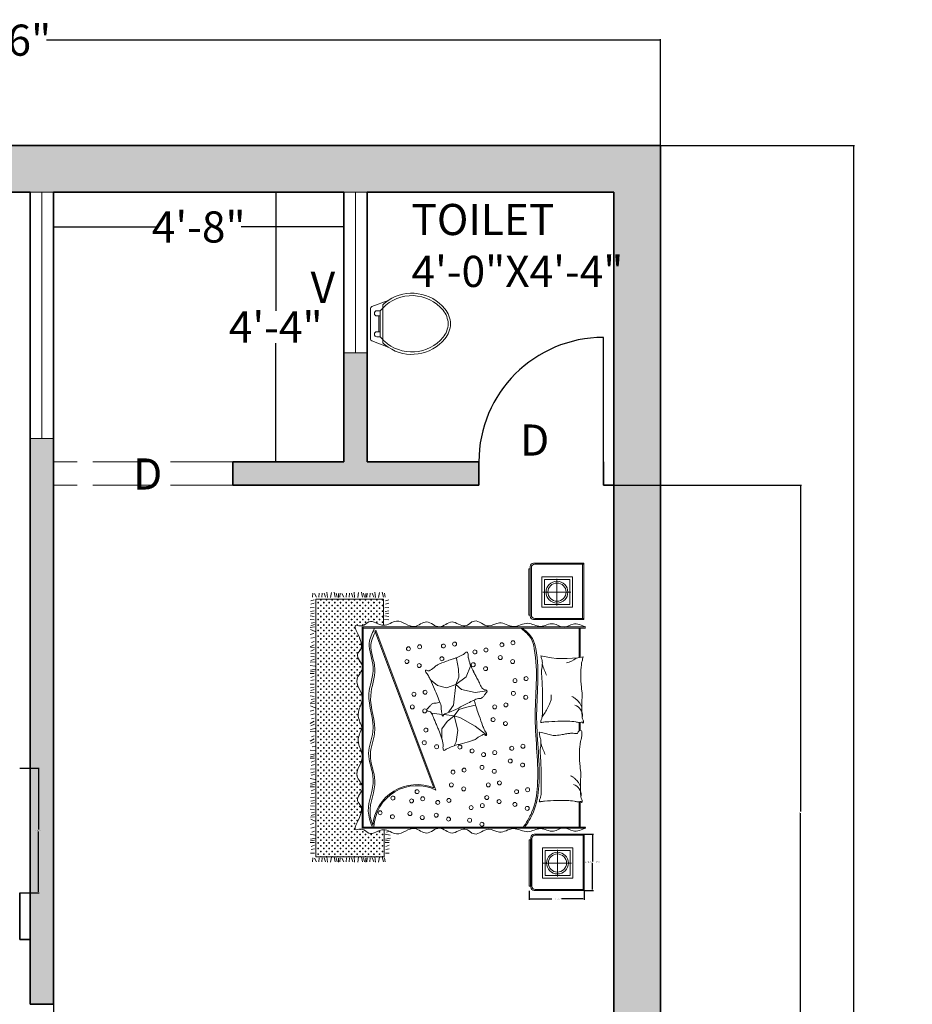
# Model space of a CAD drawing. Units: inches. Extents: x -5 to 330, y -522 to 40.
# Tile 23 of 23: x 158 to 330, y -153 to 37. Entities that reach past the tile are written whole.
import ezdxf

# ---------------------------------------------------------------- set-up
doc = ezdxf.new("R2010")
doc.units = ezdxf.units.IN
doc.header["$MEASUREMENT"] = 0
doc.linetypes.add('ACAD_ISO02W100', pattern=[15, 12, -3])
for name, color, linetype, lineweight in [('A-ANNO-DIMS', 2, 'Continuous', 18), ('A-ANNO-TEXT', 7, 'Continuous', 18), ('A-AREA-IDEN', 7, 'Continuous', 25), ('A-DOOR', 4, 'Continuous', 25), ('A-FURN', 8, 'Continuous', 18), ('A-FURN-PATT', 9, 'Continuous', 13), ('A-GLAZ', 4, 'Continuous', 18), ('A-WALL', 7, 'Continuous', 35), ('A-WALL-OVHD', 8, 'ACAD_ISO02W100', 18), ('WC-Detail_dwgmodels.com', 251, 'Continuous', 13), ('WC-Outline_dwgmodels.com', 250, 'Continuous', 18)]:
    doc.layers.add(name, color=color, linetype=linetype, lineweight=lineweight)
doc.layers.add('A-WALL-PATT', color=18, linetype='Continuous', lineweight=13, true_color=0x000000)
doc.styles.get("Standard").update_dxf_attribs({"font": 'arial.ttf'})
doc.dimstyles.get("Standard").update_dxf_attribs({"dimtxt": 0.18, "dimasz": 0.18, "dimexe": 0.18, "dimexo": 0.0625, "dimgap": 0.09, "dimtad": 0, "dimtih": 1, "dimtoh": 1, "dimdec": 0, "dimzin": 0, "dimdsep": 46, "dimlunit": 3, "dimtxsty": 'Standard', "dimcen": 0.09, "dimadec": 0, "dimazin": 0, "dimtfac": 1, "dimtdec": 0, "dimtofl": 0, "dimtmove": 0, "dimatfit": 3, "dimfxl": 1, "dimtolj": 1, "dimtzin": 0, "dimarcsym": 0})

# ---------------------------------------------------------------- blocks, each defined once
blk = doc.blocks.new('*D1')
at = {"layer": 'A-ANNO-DIMS', "color": 0, "lineweight": -2, "transparency": 16777216}
for p, q in [((23.51, 12.42), (23.51, 32.82)), ((23.69, 32.64), (141.81, 32.64)), ((280.83, 32.64), (162.71, 32.64)), ((281.01, 12.42), (281.01, 32.82))]:
    blk.add_line(p, q, dxfattribs=at)
at = {"layer": 'A-ANNO-DIMS', "color": 0, "transparency": 16777216}
for points in [[(23.69, 32.67), (23.69, 32.61), (23.51, 32.64)], [(280.83, 32.67), (280.83, 32.61), (281.01, 32.64)]]:
    blk.add_solid(points, dxfattribs=at)
at = {"layer": 'Defpoints', "color": 0, "transparency": 16777216}
for p in [(281.01, 32.64), (23.51, 12.36), (281.01, 12.36)]:
    blk.add_point(p, dxfattribs=at)
at = {"layer": 'A-ANNO-DIMS', "color": 0, "transparency": 16777216, "insert": (152.26, 32.64), "char_height": 6, "attachment_point": 5}
blk.add_mtext('\\A1;21\'-6"', dxfattribs=at)
blk = doc.blocks.new('*D6')
at = {"layer": 'A-ANNO-DIMS', "color": 0, "lineweight": -2, "transparency": 16777216}
for p, q in [((281.07, 12.36), (318.43, 12.36)), ((318.25, 12.18), (318.25, -238.29)), ((318.25, -494.96), (318.25, -244.5)), ((281.07, -495.14), (318.43, -495.14))]:
    blk.add_line(p, q, dxfattribs=at)
at = {"layer": 'A-ANNO-DIMS', "color": 0, "transparency": 16777216}
for points in [[(318.22, 12.18), (318.28, 12.18), (318.25, 12.36)], [(318.22, -494.96), (318.28, -494.96), (318.25, -495.14)]]:
    blk.add_solid(points, dxfattribs=at)
at = {"layer": 'Defpoints', "color": 0, "transparency": 16777216}
for p in [(281.01, 12.36), (281.01, -495.14), (318.25, -495.14)]:
    blk.add_point(p, dxfattribs=at)
at = {"layer": 'A-ANNO-DIMS', "color": 0, "transparency": 16777216, "insert": (318.25, -241.39), "char_height": 6, "attachment_point": 5}
blk.add_mtext('\\A1;42\'-4"', dxfattribs=at)
blk = doc.blocks.new('*D7')
at = {"layer": 'A-ANNO-DIMS', "color": 0, "lineweight": -2, "transparency": 16777216}
for p, q in [((164.01, -3.29), (164.01, -3.18)), ((164.19, -3.36), (183.82, -3.36)), ((219.83, -3.36), (200.2, -3.36)), ((220.01, -3.29), (220.01, -3.18))]:
    blk.add_line(p, q, dxfattribs=at)
at = {"layer": 'A-ANNO-DIMS', "color": 0, "transparency": 16777216}
for points in [[(164.19, -3.33), (164.19, -3.39), (164.01, -3.36)], [(219.83, -3.33), (219.83, -3.39), (220.01, -3.36)]]:
    blk.add_solid(points, dxfattribs=at)
at = {"layer": 'Defpoints', "color": 0, "transparency": 16777216}
for p in [(164.01, -3.36), (220.01, -3.36), (220.01, -3.36)]:
    blk.add_point(p, dxfattribs=at)
at = {"layer": 'A-ANNO-DIMS', "color": 0, "transparency": 16777216, "insert": (192.01, -3.36), "char_height": 6, "attachment_point": 5}
blk.add_mtext('\\A1;4\'-8"', dxfattribs=at)
blk = doc.blocks.new('*D8')
at = {"layer": 'A-ANNO-DIMS', "color": 0, "lineweight": -2, "transparency": 16777216}
for p, q in [((213.44, 3.36), (206.68, 3.36)), ((206.86, 3.18), (206.86, -19.55)), ((206.86, -48.46), (206.86, -25.73)), ((209.24, -48.64), (206.68, -48.64))]:
    blk.add_line(p, q, dxfattribs=at)
at = {"layer": 'A-ANNO-DIMS', "color": 0, "transparency": 16777216}
for points in [[(206.83, 3.18), (206.89, 3.18), (206.86, 3.36)], [(206.83, -48.46), (206.89, -48.46), (206.86, -48.64)]]:
    blk.add_solid(points, dxfattribs=at)
at = {"layer": 'Defpoints', "color": 0, "transparency": 16777216}
for p in [(213.5, 3.36), (206.86, -48.64), (209.31, -48.64)]:
    blk.add_point(p, dxfattribs=at)
at = {"layer": 'A-ANNO-DIMS', "color": 0, "transparency": 16777216, "insert": (206.86, -22.64), "char_height": 6, "attachment_point": 5}
blk.add_mtext('\\A1;4\'-4"', dxfattribs=at)
blk = doc.blocks.new('DOOR-24IN-SWING')
blk.add_line((24, 0), (24, 24))
blk.add_arc((24, 0), 24, 90, 180)
blk = doc.blocks.new('NIGHTSTAND-11IN')
for p, q in [((0.28, 10.23), (0.28, 0.65)), ((0.5, 10.01), (0.5, 0.86)), ((10.58, 10.87), (0.93, 10.87)), ((10.58, 10.66), (1.14, 10.66)), ((10.36, 0), (10.36, 10.87)), ((10.58, 0), (10.58, 10.87)), ((2.52, 8.24), (8.4, 8.24)), ((2.52, 2.36), (2.52, 8.24)), ((3.04, 7.71), (7.88, 7.71)), ((3.04, 2.88), (3.04, 7.71)), ((5.43, 2.69), (5.43, 7.83)), ((7.88, 2.88), (7.88, 7.71)), ((8.4, 2.36), (8.4, 8.24)), ((8.11, 5.29), (2.69, 5.29)), ((2.52, 2.36), (8.4, 2.36)), ((3.04, 2.88), (7.88, 2.88)), ((1.14, 0.22), (10.58, 0.22)), ((0.93, 0), (10.58, 0))]:
    blk.add_line(p, q)
blk.add_lwpolyline([(0.26, 9.8), (0.26, 0.86), (0, 0.86), (0, 9.8)], close=True)
for radius in [2.1, 1.75]:
    blk.add_circle((5.43, 5.29), radius)
for centre, start, end in [((0.93, 10.23), 90, 180), ((1.14, 10.01), 90, 180), ((0.93, 0.65), 180, 270), ((1.14, 0.86), 180, 270)]:
    blk.add_arc(centre, 0.646, start, end)
blk = doc.blocks.new('*D18')
at = {"layer": 'A-ANNO-DIMS', "color": 0, "lineweight": -2, "transparency": 16777216}
for p, q in [((157.57, -107.64), (161.29, -107.64)), ((161.11, -107.82), (161.11, -119.46)), ((161.11, -131.46), (161.11, -119.83)), ((157.57, -131.64), (161.29, -131.64))]:
    blk.add_line(p, q, dxfattribs=at)
at = {"layer": 'A-ANNO-DIMS', "color": 0, "transparency": 16777216}
for points in [[(161.08, -107.82), (161.14, -107.82), (161.11, -107.64)], [(161.08, -131.46), (161.14, -131.46), (161.11, -131.64)]]:
    blk.add_solid(points, dxfattribs=at)
at = {"layer": 'Defpoints', "color": 0, "transparency": 16777216}
for p in [(157.51, -107.64), (161.11, -107.64), (157.51, -131.64)]:
    blk.add_point(p, dxfattribs=at)
at = {"layer": 'A-ANNO-DIMS', "color": 0, "transparency": 16777216, "insert": (161.11, -119.64), "char_height": 0.18, "attachment_point": 5}
blk.add_mtext('\\A1;2\'-0" TYP.', dxfattribs=at)
blk = doc.blocks.new('*D23')
at = {"layer": 'A-ANNO-DIMS', "color": 0, "lineweight": -2, "transparency": 16777216}
for p, q in [((266.37, -120.35), (268.12, -120.35)), ((267.94, -120.53), (267.94, -125.6)), ((267.94, -131.04), (267.94, -125.97)), ((266.37, -131.22), (268.12, -131.22))]:
    blk.add_line(p, q, dxfattribs=at)
at = {"layer": 'A-ANNO-DIMS', "color": 0, "transparency": 16777216}
for points in [[(267.91, -120.53), (267.97, -120.53), (267.94, -120.35)], [(267.91, -131.04), (267.97, -131.04), (267.94, -131.22)]]:
    blk.add_solid(points, dxfattribs=at)
at = {"layer": 'Defpoints', "color": 0, "transparency": 16777216}
for p in [(266.31, -120.35), (267.94, -120.35), (266.31, -131.22)]:
    blk.add_point(p, dxfattribs=at)
at = {"layer": 'A-ANNO-DIMS', "color": 0, "transparency": 16777216, "insert": (267.94, -125.78), "char_height": 0.18, "attachment_point": 5}
blk.add_mtext('\\A1;NIGHTSTAND 0\'-11" TYP.', dxfattribs=at)
blk = doc.blocks.new('*D24')
at = {"layer": 'A-ANNO-DIMS', "color": 0, "lineweight": -2, "transparency": 16777216}
for p, q in [((255.73, -131.28), (255.73, -133.03)), ((266.31, -131.28), (266.31, -133.03)), ((255.91, -132.85), (260.1, -132.85)), ((266.13, -132.85), (261.94, -132.85))]:
    blk.add_line(p, q, dxfattribs=at)
at = {"layer": 'A-ANNO-DIMS', "color": 0, "transparency": 16777216}
for points in [[(255.91, -132.82), (255.91, -132.88), (255.73, -132.85)], [(266.13, -132.82), (266.13, -132.88), (266.31, -132.85)]]:
    blk.add_solid(points, dxfattribs=at)
at = {"layer": 'Defpoints', "color": 0, "transparency": 16777216}
for p in [(255.73, -131.22), (266.31, -131.22), (266.31, -132.85)]:
    blk.add_point(p, dxfattribs=at)
at = {"layer": 'A-ANNO-DIMS', "color": 0, "transparency": 16777216, "insert": (261.02, -132.85), "char_height": 0.18, "attachment_point": 5}
blk.add_mtext('\\A1;0\'-10 1/2" TYP.', dxfattribs=at)
blk = doc.blocks.new('*D37')
at = {"layer": 'A-ANNO-DIMS', "color": 0, "lineweight": -2, "transparency": 16777216}
for p, q in [((164.01, -53.21), (164.01, -522.31)), ((272.01, -53.21), (272.01, -522.31)), ((164.19, -522.13), (217.68, -522.13)), ((271.83, -522.13), (218.34, -522.13))]:
    blk.add_line(p, q, dxfattribs=at)
at = {"layer": 'A-ANNO-DIMS', "color": 0, "transparency": 16777216}
for points in [[(164.19, -522.1), (164.19, -522.16), (164.01, -522.13)], [(271.83, -522.1), (271.83, -522.16), (272.01, -522.13)]]:
    blk.add_solid(points, dxfattribs=at)
at = {"layer": 'Defpoints', "color": 0, "transparency": 16777216}
for p in [(164.01, -53.14), (272.01, -53.14), (272.01, -522.13)]:
    blk.add_point(p, dxfattribs=at)
at = {"layer": 'A-ANNO-DIMS', "color": 0, "transparency": 16777216, "insert": (218.01, -522.13), "char_height": 0.18, "attachment_point": 5}
blk.add_mtext('\\A1;9\'-0"', dxfattribs=at)
blk = doc.blocks.new('*D38')
at = {"layer": 'A-ANNO-DIMS', "color": 0, "lineweight": -2, "transparency": 16777216}
for p, q in [((272.07, -53.14), (308.17, -53.14)), ((307.99, -53.32), (307.99, -115.96)), ((307.99, -178.96), (307.99, -116.33)), ((272.07, -179.14), (308.17, -179.14))]:
    blk.add_line(p, q, dxfattribs=at)
at = {"layer": 'A-ANNO-DIMS', "color": 0, "transparency": 16777216}
for points in [[(307.96, -53.32), (308.02, -53.32), (307.99, -53.14)], [(307.96, -178.96), (308.02, -178.96), (307.99, -179.14)]]:
    blk.add_solid(points, dxfattribs=at)
at = {"layer": 'Defpoints', "color": 0, "transparency": 16777216}
for p in [(272.01, -53.14), (272.01, -179.14), (307.99, -179.14)]:
    blk.add_point(p, dxfattribs=at)
at = {"layer": 'A-ANNO-DIMS', "color": 0, "transparency": 16777216, "insert": (307.99, -116.14), "char_height": 0.18, "attachment_point": 5}
blk.add_mtext('\\A1;10\'-6"', dxfattribs=at)

msp = doc.modelspace()

# ---------------------------------------------------------------- hatches: boundary and pattern name
at = {"layer": 'A-FURN-PATT'}
h = msp.add_hatch(dxfattribs=at)
h.set_pattern_fill('CROSS', color=256, scale=2.153837, angle=-90, style=0)
h.set_pattern_definition([(270, (88.4915, -4740.28843), (0.538459134, -0.538459134), [0.26922957, -0.8076887]), (360, (88.35687, -4740.42304), (0.538459134, 0.538459134), [0.26922957, -0.8076887])])
edge = h.paths.add_edge_path()
edge.add_line((214.56, -124.72), (227.76, -124.72))
edge.add_line((227.76, -124.72), (227.76, -119.5))
edge.add_spline(control_points=[(227.76, -119.5), (227.72, -119.5), (226.72, -119.48), (225.06, -121.03), (223.74, -119.1), (220.78, -120.19), (224.6, -115.72), (221.98, -113.7), (223.31, -112.44), (223.51, -111.67)], knot_values=[1896.039366, 1896.039366, 1896.039366, 1896.039366, 1901.133447, 2037.052147, 2110.507177, 2158.377997, 2368.992723, 2430.676444, 2542.061162, 2542.061162, 2542.061162, 2542.061162], degree=3, periodic=0)
edge.add_line((223.51, -111.67), (223.51, -111.05))
edge.add_spline(control_points=[(223.51, -111.05), (223.34, -110.4), (221.64, -108.79), (223.28, -106.99), (223.51, -105.88)], knot_values=[2572.217644, 2572.217644, 2572.217644, 2572.217644, 2670.523569, 2827.764492, 2827.764492, 2827.764492, 2827.764492], degree=3, periodic=0)
edge.add_line((223.51, -105.88), (223.51, -104.98))
edge.add_spline(control_points=[(223.51, -104.98), (223.34, -104.08), (222.22, -102.35), (223.25, -100.64), (223.47, -99.81)], knot_values=[2870.498313, 2870.498313, 2870.498313, 2870.498313, 2999.108306, 3118.80064, 3118.80064, 3118.80064, 3118.80064], degree=3, periodic=0)
edge.add_spline(control_points=[(223.47, -99.81), (223.25, -98.97), (222.22, -97.26), (223.34, -95.53), (223.51, -94.63)], knot_values=[2870.498313, 2870.498313, 2870.498313, 2870.498313, 2990.190647, 3118.80064, 3118.80064, 3118.80064, 3118.80064], degree=3, periodic=0)
edge.add_line((223.51, -94.63), (223.51, -93.73))
edge.add_spline(control_points=[(223.51, -93.73), (223.28, -92.62), (221.64, -90.83), (223.34, -89.22), (223.51, -88.56)], knot_values=[2572.217644, 2572.217644, 2572.217644, 2572.217644, 2729.458567, 2827.764492, 2827.764492, 2827.764492, 2827.764492], degree=3, periodic=0)
edge.add_line((223.51, -88.56), (223.51, -87.95))
edge.add_spline(control_points=[(223.51, -87.95), (223.31, -87.18), (221.98, -85.91), (224.6, -83.9), (220.78, -79.43), (223.74, -80.52), (225.05, -78.59), (226.66, -80.07), (227.62, -80.11)], knot_values=[1902.697505, 1902.697505, 1902.697505, 1902.697505, 2014.082222, 2075.765943, 2286.38067, 2334.251489, 2407.70652, 2542.061162, 2542.061162, 2542.061162, 2542.061162], degree=3, periodic=0)
edge.add_line((227.62, -80.11), (227.62, -75.05))
edge.add_line((227.62, -75.05), (214.56, -75.05))
edge.add_line((214.56, -75.05), (214.56, -124.72))
at = {"layer": 'A-WALL-PATT'}
h = msp.add_hatch(color=256, dxfattribs=at)
h.dxf.hatch_style = 1
h.paths.add_polyline_path([(164.01, -44.15), (159.51, -44.15), (159.51, -153.14), (164.01, -153.14)], flags=17)
h.paths.add_polyline_path([(224.01, -188.14), (272.01, -188.14), (272.01, -218.14), (260.01, -218.14), (260.01, -222.64), (272.01, -222.64), (272.01, -292.64), (159.01, -292.64), (159.01, -297.14), (272.01, -297.14), (272.01, -417.14), (245.51, -417.14), (245.51, -426.14), (272.01, -426.14), (272.01, -495.14), (281.01, -495.14), (281.01, 12.36), (23.51, 12.36), (23.51, -426.14), (62.92, -426.14), (62.92, -417.14), (32.51, -417.14), (32.51, -297.14), (48.13, -297.14), (48.13, -292.64), (32.51, -292.64), (32.51, -140.64), (133.51, -140.64), (133.51, -131.64), (32.51, -131.64), (32.51, 3.36), (159.51, 3.36), (164.01, 3.36), (220.01, 3.36), (224.51, 3.36), (272.01, 3.36), (272.01, -179.14), (159.51, -179.14), (159.51, -188.14), (219.51, -188.14), (219.51, -266.64), (224.01, -266.64), (224.01, -222.64), (236.01, -222.64), (236.01, -218.14), (224.01, -218.14)])
h.paths.add_polyline_path([(133.01, -292.64), (128.51, -292.64), (128.51, -297.14), (128.51, -417.14), (122.92, -417.14), (122.92, -426.14), (133.01, -426.14)], flags=17)
h.paths.add_polyline_path([(185.51, -417.14), (159.01, -417.14), (159.01, -426.14), (185.51, -426.14)], flags=17)
h.paths.add_polyline_path([(133.51, -140.64), (129.01, -140.64), (129.01, -246.64), (133.51, -246.64)], flags=17)
h.paths.add_polyline_path([(246.01, -48.64), (224.51, -48.64), (224.51, -27.63), (220.01, -27.63), (220.01, -48.64), (198.6, -48.64), (198.6, -53.14), (246.01, -53.14)], flags=17)

# ---------------------------------------------------------------- linework, layer by layer
at = {"layer": 'A-FURN'}
for p, q in [((213.96, -74.66), (214.03, -73.93)), ((214.71, -74.66), (214.34, -73.99)), ((215.16, -74.66), (215.23, -73.93)), ((215.73, -74.66), (215.8, -73.93)), ((216.48, -74.66), (216.21, -73.93)), ((216.81, -74.77), (216.72, -73.75)), ((217.42, -74.77), (217.58, -73.81)), ((218.33, -74.71), (218.13, -73.75)), ((218.69, -74.71), (218.54, -73.93)), ((218.99, -74.77), (218.99, -73.97)), ((219.22, -74.66), (219.29, -73.93)), ((219.97, -74.66), (219.59, -73.99)), ((220.41, -74.66), (220.48, -73.93)), ((220.99, -74.66), (221.06, -73.93)), ((221.74, -74.66), (221.47, -73.93)), ((222.07, -74.77), (221.97, -73.75)), ((222.68, -74.77), (222.84, -73.81)), ((223.59, -74.71), (223.39, -73.75)), ((223.94, -74.71), (223.8, -73.93)), ((224.25, -74.77), (224.25, -73.97)), ((224.43, -74.66), (224.5, -73.93)), ((225.01, -74.66), (225.08, -73.93)), ((225.76, -74.66), (225.48, -73.93)), ((226.09, -74.77), (225.99, -73.75)), ((226.7, -74.77), (226.85, -73.81)), ((227.61, -74.71), (227.4, -73.75)), ((227.96, -74.71), (227.81, -73.93)), ((213.65, -75.43), (214.29, -75.18)), ((213.65, -76.04), (214.29, -75.87)), ((214.56, -75.05), (214.56, -124.72)), ((227.62, -75.05), (214.56, -75.05)), ((227.62, -80.11), (227.62, -75.05)), ((227.99, -75.43), (228.63, -75.18)), ((227.99, -76.04), (228.63, -75.87)), ((213.53, -76.75), (214.29, -76.71)), ((213.59, -77.45), (214.29, -77.31)), ((213.65, -77.91), (214.29, -77.77)), ((227.88, -76.75), (228.63, -76.71)), ((227.93, -77.45), (228.63, -77.31)), ((227.99, -77.91), (228.63, -77.77)), ((213.48, -78.97), (214.29, -79.09)), ((213.53, -78.31), (214.29, -78.42)), ((213.71, -79.68), (214.32, -79.58)), ((227.82, -78.97), (228.63, -79.09)), ((227.88, -78.31), (228.63, -78.42)), ((213.53, -80.54), (214.32, -80.44)), ((213.59, -80.89), (214.43, -81.3)), ((213.65, -80.23), (214.32, -79.98)), ((266.59, -80.42), (223.51, -80.42)), ((223.51, -80.42), (223.51, -119.19)), ((266.59, -80.64), (223.51, -80.64)), ((223.73, -80.42), (223.73, -119.19)), ((225.98, -81.15), (237.33, -111.45)), ((226.18, -81.08), (237.71, -111.86)), ((265.35, -80.64), (265.35, -86.32)), ((265.56, -80.64), (265.56, -86.29)), ((213.53, -81.91), (214.2, -81.7)), ((213.6, -82.62), (214.31, -82.47)), ((213.76, -83.43), (214.29, -83.24)), ((213.53, -84.27), (214.29, -83.85)), ((213.6, -84.37), (214.32, -84.44)), ((213.6, -85.12), (214.26, -84.75)), ((213.48, -87.23), (214.5, -87.13)), ((213.6, -85.57), (214.32, -85.64)), ((213.6, -86.15), (214.32, -86.22)), ((213.6, -86.9), (214.32, -86.62)), ((241.71, -86.48), (241.57, -86.41)), ((242.08, -88.59), (241.71, -86.48)), ((213.48, -87.84), (214.44, -87.99)), ((213.54, -88.75), (214.5, -88.54)), ((213.54, -89.1), (214.32, -88.95)), ((242.15, -90.08), (242.08, -88.59)), ((243.56, -90.04), (244.38, -88)), ((244.38, -88), (244.3, -87.48)), ((213.48, -89.4), (214.29, -89.4)), ((213.65, -90.17), (214.29, -89.92)), ((213.65, -90.77), (214.29, -90.6)), ((238.01, -91.74), (236.66, -90.59)), ((241.56, -91.52), (243.56, -90.04)), ((241.56, -91.52), (242.15, -90.08)), ((213.53, -91.48), (214.29, -91.44)), ((213.59, -92.19), (214.29, -92.04)), ((213.65, -92.65), (214.29, -92.5)), ((239.78, -92.19), (238.01, -91.74)), ((241.56, -91.52), (239.78, -92.19)), ((241.56, -91.52), (241.15, -95.52)), ((242.67, -92.48), (241.56, -91.52)), ((245.3, -93.04), (242.67, -92.48)), ((247.52, -92.74), (245.3, -93.04)), ((213.48, -93.7), (214.29, -93.82)), ((213.53, -93.05), (214.29, -93.15)), ((213.65, -94.97), (214.32, -94.71)), ((213.71, -94.42), (214.32, -94.31)), ((213.53, -95.27), (214.32, -95.17)), ((213.53, -96.64), (214.2, -96.44)), ((213.59, -95.63), (214.43, -96.04)), ((240.38, -96.6), (240.19, -96.86)), ((241.58, -96.32), (240.37, -96.82)), ((241.15, -95.52), (240.38, -96.6)), ((241.28, -97.58), (242.17, -96.34)), ((242.17, -96.34), (243.41, -95.92)), ((243.41, -95.92), (245.32, -95.49)), ((213.53, -99.01), (214.29, -98.59)), ((213.6, -97.36), (214.31, -97.2)), ((213.76, -98.16), (214.29, -97.98)), ((238.94, -97.28), (236.9, -97.03)), ((239.92, -98.64), (238.9, -100.05)), ((241.28, -97.58), (239.25, -97.32)), ((240.37, -96.82), (239.43, -97.2)), ((241.28, -97.58), (239.92, -98.64)), ((241.28, -97.58), (241.96, -100.35)), ((242.47, -97.96), (241.28, -97.58)), ((245.28, -99.58), (242.47, -97.96)), ((213.59, -100.17), (214.49, -99.97)), ((213.6, -99.5), (214.32, -99.16)), ((238.9, -100.05), (238.9, -102.05)), ((241.96, -100.35), (241.66, -102.56)), ((247.52, -101.28), (245.28, -99.58)), ((265.35, -98.85), (265.35, -100.43)), ((265.56, -98.85), (265.56, -100.35)), ((213.53, -100.57), (214.43, -100.67)), ((213.53, -102.43), (214.29, -102.01)), ((213.76, -101.58), (214.29, -101.4)), ((257.68, -100.7), (258.32, -100.86)), ((258.32, -100.86), (260.1, -101.3)), ((213.51, -104.17), (214.47, -104.33)), ((213.6, -102.92), (214.32, -102.58)), ((213.88, -103.53), (214.49, -103.39)), ((241.66, -102.56), (241.23, -103.34)), ((213.51, -105.74), (214.32, -105.74)), ((213.57, -105.09), (214.53, -104.88)), ((213.57, -105.44), (214.35, -105.29)), ((213.56, -107.82), (214.32, -107.78)), ((213.68, -106.51), (214.32, -106.25)), ((213.68, -107.11), (214.32, -106.94)), ((213.51, -109.66), (214.47, -109.82)), ((213.62, -108.52), (214.32, -108.38)), ((213.68, -108.98), (214.32, -108.84)), ((213.51, -111.23), (214.32, -111.23)), ((213.57, -110.57), (214.53, -110.36)), ((213.57, -110.92), (214.35, -110.78)), ((213.68, -111.99), (214.32, -111.74)), ((213.56, -113.3), (214.32, -113.26)), ((213.68, -112.6), (214.32, -112.43)), ((213.5, -115.53), (214.32, -115.65)), ((213.56, -114.87), (214.32, -114.97)), ((213.62, -114.01), (214.32, -113.87)), ((213.68, -114.47), (214.32, -114.32)), ((265.35, -114.12), (265.35, -118.98)), ((265.56, -114.06), (265.56, -118.98)), ((213.56, -117.1), (214.35, -117)), ((213.62, -117.45), (214.46, -117.86)), ((213.68, -116.79), (214.35, -116.54)), ((213.73, -116.24), (214.35, -116.14)), ((213.56, -118.47), (214.23, -118.26)), ((213.63, -119.18), (214.34, -119.03)), ((266.59, -118.98), (223.51, -118.98)), ((266.59, -119.19), (223.51, -119.19)), ((227.76, -124.72), (227.76, -119.5)), ((213.51, -120.39), (214.47, -120.55)), ((213.57, -121.3), (214.53, -121.1)), ((213.79, -119.98), (214.32, -119.8)), ((227.95, -120.39), (228.91, -120.55)), ((228.01, -121.3), (228.97, -121.1)), ((228.23, -119.98), (228.75, -119.8)), ((213.51, -121.96), (214.32, -121.96)), ((213.57, -121.65), (214.35, -121.51)), ((213.68, -122.72), (214.32, -122.47)), ((213.68, -123.33), (214.32, -123.16)), ((227.95, -121.96), (228.75, -121.96)), ((228.01, -121.65), (228.79, -121.51)), ((228.11, -122.72), (228.75, -122.47)), ((228.11, -123.33), (228.75, -123.16)), ((213.56, -124.04), (214.32, -124)), ((213.96, -125.66), (214.03, -124.93)), ((214.71, -125.66), (214.34, -124.99)), ((214.56, -124.72), (227.76, -124.72)), ((215.16, -125.66), (215.23, -124.93)), ((215.73, -125.66), (215.8, -124.93)), ((216.48, -125.66), (216.21, -124.93)), ((216.81, -125.77), (216.72, -124.75)), ((217.42, -125.77), (217.58, -124.81)), ((218.33, -125.71), (218.13, -124.75)), ((218.69, -125.71), (218.54, -124.93)), ((218.99, -125.77), (218.99, -124.97)), ((219.22, -125.66), (219.29, -124.93)), ((219.97, -125.66), (219.59, -124.99)), ((220.41, -125.66), (220.48, -124.93)), ((220.99, -125.66), (221.06, -124.93)), ((221.74, -125.66), (221.47, -124.93)), ((222.07, -125.77), (221.97, -124.75)), ((222.68, -125.77), (222.84, -124.81)), ((223.59, -125.71), (223.39, -124.75)), ((223.94, -125.71), (223.8, -124.93)), ((224.25, -125.77), (224.25, -124.97)), ((224.43, -125.66), (224.5, -124.93)), ((225.01, -125.66), (225.08, -124.93)), ((225.76, -125.66), (225.48, -124.93)), ((226.09, -125.77), (225.99, -124.75)), ((226.7, -125.77), (226.85, -124.81)), ((227.61, -125.71), (227.4, -124.75)), ((227.96, -125.71), (227.81, -124.93)), ((228, -124.04), (228.75, -124))]:
    msp.add_line(p, q, dxfattribs=at)
for centre in [(241.33, -83.72), (252.59, -83.49), (232.44, -84.64), (234.59, -84.26), (239.19, -84.1), (245.24, -85.25), (247.38, -84.87), (250.45, -83.87), (232.14, -87.09), (238.88, -86.56), (250.14, -86.33), (252.52, -87.09), (234.51, -87.86), (244.93, -87.71), (247.31, -88.47), (252.98, -90.77), (255.12, -90.39), (235.65, -93), (252.67, -93.23), (233.5, -93.39), (255.05, -93.99), (233.19, -95.84), (235.57, -96.61), (249.07, -95.83), (251.22, -95.45), (248.76, -98.29), (235.8, -100.29), (251.14, -99.05), (235.49, -102.74), (237.87, -103.51), (242.35, -103.57), (244.72, -104.33), (249.07, -104.65), (252.36, -103.81), (254.51, -103.42), (246.92, -105.03), (252.06, -106.26), (241.03, -108.41), (243.17, -108.02), (246.62, -107.49), (248.99, -108.25), (254.43, -107.03), (234.11, -112.17), (240.72, -110.86), (243.09, -111.63), (247.84, -110.86), (249.99, -110.48), (253.27, -112.17), (255.41, -111.79), (229.44, -113.4), (233.04, -113.94), (235.19, -113.55), (240.24, -113.86), (247.54, -113.31), (249.91, -114.08), (238.1, -114.24), (244.53, -115.24), (246.68, -114.86), (252.96, -114.63), (255.34, -115.39), (226.99, -116.24), (229.36, -117), (232.73, -116.39), (235.11, -117.16), (237.79, -116.7), (240.17, -117.46), (244.23, -117.69), (246.6, -118.46)]:
    msp.add_circle(centre, 0.383, dxfattribs=at)
for centre, radius, start, end in [((243.68, -85.62), 0.361, 89.0386, 139.4914), ((243.69, -85.39), 0.125, 31.6917, 89.0386), ((242.86, -85.9), 1.1, 13.0402, 31.6917), ((254.77, -127.49), 43.14, 109.6584, 112.2355), ((252.2, -120.29), 35.5, 108.2369, 109.6584), ((237.42, -75.42), 11.75, 288.2369, 290.7081), ((240.2, -82.79), 3.87, 290.7081, 295.1732), ((217.46, -34.41), 57.33, 295.1732, 296.3332), ((242.17, -84.33), 1.63, 296.3332, 319.4914), ((242.67, -85.94), 1.29, 356.6119, 13.0402), ((245.31, -86.1), 1.36, 176.6119, 192.6252), ((253.03, -84.37), 9.26, 192.6252, 200.7486), ((262.49, -67.94), 18.6, 255.9578, 281.1903), ((262.85, -85.17), 4.95, 189.4841, 197.3864), ((255.67, -87.42), 2.58, 6.4341, 17.3864), ((255.11, -87.48), 3.14, 348.4414, 6.4341), ((262.61, -84.32), 3.01, 275.6311, 315.0976), ((270.94, -88.42), 5.22, 164.256, 172.4531), ((259.6, -85.23), 6.56, 344.256, 351.5628), ((235.83, -88.82), 0.0955, 107.6767, 180.4475), ((236.5, -88.81), 0.759, 180.4475, 204.7411), ((235.84, -88.86), 0.136, 40.9751, 107.6767), ((236.98, -88.59), 1.3, 204.7411, 222.9813), ((236.18, -88.57), 0.305, 220.9751, 263.9885), ((236.32, -87.22), 1.66, 263.9885, 271.6673), ((236.36, -88.55), 0.329, 271.6673, 288.9668), ((236.19, -88.06), 0.847, 288.9668, 301.2138), ((232.7, -82.3), 7.58, 301.2138, 305.3015), ((234.67, -85.08), 4.18, 305.3015, 314.0964), ((238.79, -89.33), 1.74, 120.4694, 134.0964), ((240.05, -91.48), 4.23, 112.2355, 120.4694), ((256.93, -82.89), 13.43, 200.7486, 207.4921), ((356.56, -31.04), 125.75, 207.4921, 207.8482), ((263.04, -89.11), 4.95, 168.4414, 182.7491), ((273.45, -82.95), 15.91, 197.1982, 205.3111), ((280.35, -89.67), 14.7, 172.4531, 180), ((234.79, -90.64), 1.71, 27.1028, 42.9813), ((220.26, -98.07), 18.03, 24.5246, 27.1028), ((136.84, -136.13), 109.72, 23.4795, 24.5246), ((129.17, -151.18), 131.42, 27.4999, 27.8482), ((207.23, -110.54), 43.43, 26.4147, 27.4999), ((288.32, -87.89), 30.26, 182.7491, 184.6176), ((232.04, -92.44), 26.2, 2.6096, 4.6176), ((288.24, -89.67), 22.59, 180, 186.0867), ((175.34, -119.41), 67.74, 21.0043, 23.4795), ((305.86, -61.55), 66.71, 206.4147, 207.2902), ((247.27, -91.78), 0.772, 207.2902, 273.2455), ((247.33, -92.83), 0.274, 321.1864, 93.2455), ((185.87, -94.54), 72.42, 0.9704, 2.6096), ((277.11, -90.86), 11.4, 186.0867, 190.1899), ((262.66, -93.45), 3.28, 2.5386, 10.1899), ((260.15, -127.6), 36.33, 115.0529, 117.0884), ((253.94, -114.3), 21.66, 112.4162, 115.0529), ((247.57, -94.06), 2.51, 190.7366, 196.6085), ((310.08, -75.42), 67.74, 196.6085, 199.0836), ((246.06, -95.2), 0.987, 81.9508, 112.4162), ((246.26, -93.74), 0.487, 261.9508, 305.8936), ((245.57, -92.78), 1.67, 305.8936, 316.4776), ((243.38, -90.7), 4.69, 316.4776, 322.7849), ((235.78, -84.93), 14.23, 322.7849, 323.7837), ((253.91, -98.2), 8.24, 142.4713, 143.7837), ((248.15, -93.78), 0.974, 135.8726, 142.4713), ((246.37, -92.06), 1.5, 315.8726, 321.1864), ((135.13, -95.4), 123.17, 359.7135, 0.9704), ((249.66, -90.79), 10.91, 335.6735, 339.3257), ((258.7, -94.2), 1.25, 339.3257, 355.9172), ((254.11, -93.87), 5.86, 355.9172, 3.5552), ((262.27, -97.8), 4.31, 61.6832, 66.9972), ((263.81, -94.94), 1.06, 50.9651, 61.6832), ((261.43, -97.89), 4.85, 43.8115, 50.9651), ((258.84, -100.37), 8.44, 38.3886, 43.8115), ((284.66, -95.68), 18.81, 175.1982, 179.4243), ((259.7, -93.58), 6.24, 355.1982, 2.5386), ((236.27, -96.4), 0.274, 136.7905, 268.8496), ((237.17, -97.24), 1.5, 131.4767, 136.7905), ((235.53, -95.39), 0.974, 311.4767, 318.0754), ((230.12, -90.53), 8.24, 318.0754, 319.3878), ((236.25, -97.45), 0.772, 22.8944, 88.8496), ((247.18, -105.16), 14.23, 138.389, 139.3878), ((240.04, -98.82), 4.69, 132.0817, 138.389), ((238.02, -96.58), 1.67, 121.4977, 132.0817), ((237.4, -95.58), 0.487, 77.5549, 121.4977), ((237.72, -94.14), 0.987, 257.5549, 288.0203), ((231.33, -74.48), 21.66, 288.0203, 289.3448), ((236.24, -96.03), 2.51, 8.1216, 21.0043), ((237.31, -95.87), 1.43, 355.4882, 8.1216), ((240.26, -96.11), 1.53, 175.4882, 187.6784), ((242.57, -95.79), 3.86, 187.6784, 194.8807), ((239.83, -92.05), 4.62, 292.2355, 299.936), ((258.96, -125.27), 33.71, 117.0884, 119.936), ((233.23, -95.89), 25.07, 356.426, 359.7135), ((253.08, -93.34), 6.73, 327.865, 333.5015), ((231.5, -82.58), 30.85, 333.5015, 335.6735), ((263.85, -97.52), 2.14, 355.7841, 71.5603), ((264.15, -96.16), 1.65, 27.2396, 38.3886), ((261.14, -97.71), 5.04, 20.8603, 27.2396), ((298.04, -95.82), 32.18, 179.4243, 181.9079), ((175.51, -123.1), 66.71, 22.0188, 22.8944), ((277.61, -81.81), 43.43, 202.0188, 203.104), ((234.77, -97.87), 4.21, 7.9822, 14.8807), ((238.21, -97.38), 0.732, 355.7407, 7.9822), ((239.14, -97.45), 0.198, 175.7407, 199.3799), ((239.05, -97.49), 0.101, 199.3799, 342.8133), ((239.62, -97.66), 0.497, 112.2355, 162.8133), ((349.76, -61.69), 109.72, 199.0836, 200.1287), ((259.78, -99.01), 1.88, 163.7788, 172.8796), ((259.56, -98.95), 1.65, 152.7159, 163.7788), ((257.22, -97.74), 0.975, 332.7159, 347.131), ((255.11, -97.26), 3.14, 347.131, 356.426), ((245.49, -88.57), 15.69, 324.1737, 327.865), ((276.86, -391.87), 293.69, 93.055, 93.5049), ((262.77, -127.96), 29.4, 91.6331, 93.055), ((262.35, -113.18), 14.62, 86.6313, 91.6331), ((262.05, -118.22), 19.67, 82.3191, 86.6313), ((283.54, -96.3), 17.68, 181.9079, 185.2592), ((267.09, -97.81), 1.16, 185.2592, 210.6513), ((265.56, -98.72), 0.622, 355.6975, 30.6513), ((358.55, -47.28), 131.42, 203.104, 203.4523), ((122.62, -149.63), 125.75, 23.0962, 23.4523), ((225.94, -105.57), 13.43, 16.3527, 23.0962), ((263.66, -93.25), 18.03, 200.1287, 202.7069), ((248.61, -99.55), 1.71, 202.7069, 218.5854), ((257.94, -98.78), 0.0285, 172.8796, 253.3022), ((258.05, -98.41), 0.416, 253.3022, 279.9984), ((259.33, -105.63), 6.92, 93.5049, 99.9984), ((264.11, -102.96), 4.27, 77.8905, 82.3191), ((266.12, -93.6), 5.3, 257.8905, 261.8665), ((265.77, -101.04), 0.736, 116.5805, 175.5998), ((265.47, -98.15), 0.706, 261.8665, 291.421), ((265.56, -100.63), 0.283, 11.2724, 116.5805), ((265.85, -99.12), 0.336, 68.0096, 111.421), ((265.94, -98.89), 0.0922, 348.1069, 68.0096), ((266.08, -98.92), 0.0499, 168.1069, 289.564), ((266.07, -98.9), 0.0737, 289.564, 338.2117), ((265.64, -98.73), 0.541, 338.2117, 355.6975), ((229.94, -104.4), 9.26, 8.2293, 16.3527), ((231.5, -61.27), 43.14, 285.2625, 287.8396), ((243.42, -98.3), 4.23, 287.8396, 296.0735), ((244.52, -100.54), 1.74, 296.0735, 309.7005), ((248.3, -105.1), 4.18, 120.9056, 129.7005), ((250.05, -108.02), 7.58, 116.8179, 120.9056), ((247.01, -102.01), 0.847, 104.5709, 116.8179), ((246.88, -101.5), 0.329, 87.2714, 104.5709), ((246.82, -102.84), 1.66, 79.5926, 87.2714), ((247.06, -101.5), 0.305, 36.5792, 79.5926), ((246.26, -101.42), 1.3, 20.3452, 38.5854), ((247.41, -101.24), 0.136, 216.5792, 356.0476), ((246.76, -101.23), 0.759, 356.0516, 20.3452), ((257.67, -100.72), 0.0197, 75.9551, 184.0829), ((263.47, -100.3), 5.83, 184.0829, 189.4841), ((262.6, -100.45), 4.95, 189.4841, 197.3864), ((255.41, -102.7), 2.58, 6.4341, 17.3864), ((254.85, -102.76), 3.14, 348.4414, 6.4341), ((260.46, -99.89), 1.46, 255.9548, 272.6649), ((259.86, -87.17), 14.19, 272.6649, 278.0051), ((260.89, -94.46), 6.83, 278.0051, 282.1984), ((266.35, -119.7), 19, 99.6844, 102.1984), ((263.89, -105.31), 4.39, 90, 99.6844), ((263.89, -111.51), 10.59, 83.7676, 90), ((270.69, -103.7), 5.22, 164.256, 172.4531), ((259.35, -100.5), 6.56, 344.256, 351.5628), ((263.93, -100.96), 1.95, 0, 11.2724), ((262.41, -100.96), 3.47, 351.5628, 0), ((240.38, -103.62), 1.29, 172.216, 188.6443), ((237.76, -103.27), 1.36, 352.216, 8.2293), ((240.19, -103.65), 1.1, 188.6443, 207.2959), ((239.33, -104.1), 0.125, 207.2959, 264.6428), ((239.35, -103.86), 0.361, 264.6428, 315.0955), ((240.76, -105.27), 1.63, 111.9373, 135.0955), ((261.57, -156.94), 57.33, 110.7773, 111.9373), ((242.61, -106.95), 3.87, 106.3122, 110.7773), ((244.82, -114.51), 11.75, 103.841, 106.3122), ((233.52, -68.64), 35.5, 283.841, 285.2625), ((262.79, -104.38), 4.95, 168.4414, 182.7491), ((273.19, -98.22), 15.91, 197.1982, 205.3111), ((280.09, -104.95), 14.7, 172.4531, 180), ((288.06, -103.17), 30.26, 182.7491, 184.6176), ((231.79, -107.71), 26.2, 2.6096, 4.6176), ((287.98, -104.95), 22.59, 180, 186.0867), ((185.62, -109.82), 72.42, 0.9704, 2.6096), ((276.85, -106.13), 11.4, 186.0867, 190.1899), ((134.87, -110.68), 123.17, 359.7135, 0.9704), ((262.01, -113.08), 4.31, 61.6832, 66.9972), ((263.56, -110.22), 1.06, 50.9651, 61.6832), ((261.17, -113.16), 4.85, 43.8115, 50.9651), ((258.58, -115.64), 8.44, 38.3886, 43.8115), ((284.4, -110.96), 18.81, 175.1982, 179.4243), ((262.4, -108.73), 3.28, 2.5386, 10.1899), ((259.45, -108.86), 6.24, 355.1982, 2.5386), ((234.07, -119.3), 8.5, 67.4442, 175.7493), ((234.07, -119.3), 8.29, 63.9063, 177.7674), ((232.97, -111.17), 25.07, 356.426, 359.7135), ((263.59, -112.8), 2.14, 355.7841, 71.5603), ((263.9, -111.43), 1.65, 27.2396, 38.3886), ((260.89, -112.98), 5.04, 20.8603, 27.2396), ((297.78, -111.09), 32.18, 179.4243, 181.9079), ((259.53, -114.29), 1.88, 163.7788, 172.8796), ((259.3, -114.22), 1.65, 152.7159, 163.7788), ((256.97, -113.02), 0.975, 332.7159, 347.131), ((254.86, -112.54), 3.14, 347.131, 356.426), ((283.28, -111.57), 17.68, 181.9079, 185.2592), ((266.84, -113.09), 1.16, 185.2592, 210.6513), ((265.3, -114), 0.622, 355.6975, 30.6513), ((257.68, -114.06), 0.0285, 172.8796, 253.3022), ((257.8, -113.69), 0.416, 253.3022, 279.9984), ((259.07, -120.91), 6.92, 93.5049, 99.9984), ((276.6, -407.14), 293.69, 93.055, 93.5049), ((262.52, -143.24), 29.4, 91.6331, 93.055), ((262.09, -128.46), 14.62, 86.6313, 91.6331), ((261.8, -133.49), 19.67, 82.3191, 86.6313), ((263.86, -118.24), 4.27, 77.8905, 82.3191), ((265.86, -108.88), 5.3, 257.8905, 261.8665), ((265.21, -113.43), 0.706, 261.8665, 291.421), ((265.59, -114.4), 0.336, 68.0096, 111.421), ((265.68, -114.17), 0.0922, 348.1069, 68.0096), ((265.82, -114.2), 0.0499, 168.1069, 289.564), ((265.82, -114.18), 0.0737, 289.564, 338.2117), ((265.38, -114), 0.541, 338.2117, 355.6975)]:
    msp.add_arc(centre, radius, start, end, dxfattribs=at)
for points, knots in [([(266.66, -80.5), (265.82, -80.1), (264.39, -79.41), (262.33, -81.02), (260.28, -79.18), (257.89, -80.92), (255.35, -79.09), (252.67, -81.04), (250.15, -78.99), (247.66, -81.02), (245.35, -78.36), (243.22, -81.08), (240.81, -78.55), (238.42, -81.34), (235.98, -78.61), (233.28, -81.34), (230.43, -78.33), (227.63, -80.98), (225.06, -78.58), (223.74, -80.52), (220.78, -79.43), (224.6, -83.9), (221.9, -85.98), (224.52, -88.22), (221.43, -90.79), (224.58, -93.93), (222.09, -97.06), (223.25, -98.97), (223.47, -99.81)], [0, 0, 0, 0, 119.23822, 203.934156, 305.051348, 423.414205, 538.771408, 673.601551, 801.564672, 901.488314, 1036.739405, 1131.503109, 1252.869042, 1373.114912, 1497.089457, 1612.174498, 1779.078494, 1901.133447, 2037.052147, 2110.507177, 2158.377997, 2368.992723, 2430.676444, 2554.510696, 2670.523569, 2841.287389, 2999.108306, 3118.80064, 3118.80064, 3118.80064, 3118.80064]), ([(225.84, -80.81), (225.41, -81.71), (224.26, -84.07), (226.46, -88.36), (223.81, -94), (226.55, -99.62), (224.02, -105.04), (226.65, -110.14), (224.04, -114.97), (225.1, -117.97), (225.49, -118.98)], [0, 0, 0, 0, 134.096191, 351.943146, 593.51487, 936.925241, 1129.231545, 1368.385454, 1657.415202, 1803.02854, 1803.02854, 1803.02854, 1803.02854]), ([(226.17, -81.12), (225.74, -82.02), (224.59, -84.38), (226.8, -88.66), (224.14, -94.31), (226.88, -99.93), (224.35, -105.35), (226.98, -110.44), (224.49, -115.06), (225.3, -117.87), (225.59, -118.67)], [0, 0, 0, 0, 134.096191, 351.943146, 593.51487, 936.925241, 1129.231545, 1368.385454, 1657.415202, 1773.3935, 1773.3935, 1773.3935, 1773.3935]), ([(254.22, -80.74), (254.93, -81.32), (256.18, -82.36), (257.64, -88.42), (256.16, -97.93), (257.88, -108.39), (256.72, -115.72), (255.14, -118.16), (254.49, -119.16)], [0, 0, 0, 0, 2.673077, 4.702769, 18.155955, 31.175796, 36.297027, 39.840606, 39.840606, 39.840606, 39.840606]), ([(254.51, -80.74), (255.22, -81.32), (256.47, -82.36), (257.92, -88.42), (256.44, -97.93), (258.16, -108.39), (257.01, -115.72), (255.42, -118.16), (254.78, -119.16)], [0, 0, 0, 0, 2.673077, 4.702769, 18.155955, 31.175796, 36.297027, 39.840606, 39.840606, 39.840606, 39.840606]), ([(266.66, -119.12), (265.82, -119.52), (264.39, -120.21), (262.33, -118.59), (260.28, -120.43), (257.89, -118.69), (255.35, -120.53), (252.67, -118.58), (250.15, -120.63), (247.66, -118.6), (245.35, -121.25), (243.22, -118.53), (240.81, -121.07), (238.42, -118.27), (235.98, -121), (233.28, -118.27), (230.43, -121.28), (227.63, -118.64), (225.06, -121.03), (223.74, -119.1), (220.78, -120.19), (224.6, -115.72), (221.9, -113.63), (224.52, -111.39), (221.43, -108.83), (224.58, -105.68), (222.09, -102.55), (223.25, -100.64), (223.47, -99.81)], [0, 0, 0, 0, 119.23822, 203.934156, 305.051348, 423.414205, 538.771408, 673.601551, 801.564672, 901.488314, 1036.739405, 1131.503109, 1252.869042, 1373.114912, 1497.089457, 1612.174498, 1779.078494, 1901.133447, 2037.052147, 2110.507177, 2158.377997, 2368.992723, 2430.676444, 2554.510696, 2670.523569, 2841.287389, 2999.108306, 3118.80064, 3118.80064, 3118.80064, 3118.80064])]:
    msp.add_open_spline(points, degree=3, knots=knots, dxfattribs=at)
at = {"layer": 'A-GLAZ'}
for p, q in [((159.51, 3.36), (164.01, 3.36)), ((161.76, 3.36), (161.76, -44.15)), ((220.01, 3.36), (224.51, 3.36)), ((222.26, 3.36), (222.26, -27.63)), ((220.01, -27.63), (224.51, -27.63)), ((164.01, -44.15), (159.51, -44.15))]:
    msp.add_line(p, q, dxfattribs=at)
at = {"layer": 'A-WALL'}
for p, q in [((23.51, 12.36), (281.01, 12.36)), ((281.01, 12.36), (281.01, -495.14)), ((32.51, 3.36), (159.51, 3.36)), ((159.51, 3.36), (159.51, -153.14)), ((164.01, 3.36), (164.01, -153.14)), ((164.01, 3.36), (220.01, 3.36)), ((220.01, 3.36), (220.01, -48.64)), ((224.51, 3.36), (224.51, -48.64)), ((224.51, 3.36), (272.01, 3.36)), ((272.01, 3.36), (272.01, -179.14)), ((198.6, -48.64), (220.01, -48.64)), ((198.6, -48.64), (198.6, -53.14)), ((224.51, -48.64), (246.01, -48.64)), ((246.01, -53.14), (246.01, -48.64)), ((270.01, -53.14), (270.01, -48.64)), ((198.6, -53.14), (246.01, -53.14)), ((270.01, -53.14), (272.01, -53.14)), ((157.51, -140.64), (157.51, -131.64)), ((157.51, -140.64), (159.51, -140.64)), ((159.51, -153.14), (164.01, -153.14))]:
    msp.add_line(p, q, dxfattribs=at)
at = {"layer": 'A-WALL-OVHD'}
for p, q in [((198.6, -48.64), (164.01, -48.64)), ((198.6, -53.14), (164.01, -53.14))]:
    msp.add_line(p, q, dxfattribs=at)
at = {"layer": 'WC-Detail_dwgmodels.com'}
for p, q in [((227.48, -18.98), (227.48, -18.33)), ((227.48, -25.7), (227.48, -25.05))]:
    msp.add_line(p, q, dxfattribs=at)
for points in [[(227.48, -18.33, -0.040937), (228.54, -17.5, -0.163732)], [(227.02, -19.51), (226.37, -19.51, 1), (226.37, -20.5), (226.71, -20.5)], [(227.02, -19.51, -0.022712), (227.48, -18.98, -0.162618)], [(227.02, -22.02), (227.02, -19.51, -0.476108)], [(227.02, -22.02), (227.02, -24.52, 0.022712)], [(227.02, -24.52), (226.37, -24.52, -1), (226.37, -23.54), (226.71, -23.54)], [(227.02, -24.52, 0.022712), (227.48, -25.05, 0.162618)], [(227.48, -25.7, 0.040937), (228.54, -26.53, 0.163732)]]:
    msp.add_lwpolyline(points, format="xyb", dxfattribs=at)
for points in [[(226.71, -20.5), (226.71, -23.54)], [(226.71, -20.5), (227.02, -20.5)], [(226.71, -23.54), (227.02, -23.54)]]:
    msp.add_lwpolyline(points, dxfattribs=at)
at = {"layer": 'WC-Outline_dwgmodels.com'}
for p in [(227.48, -18.98), (227.48, -25.05)]:
    msp.add_line(p, (227.48, -22.02), dxfattribs=at)
for points in [[(227.48, -18.98, -0.448546), (239.11, -19.41, -0.162618), (240.11, -22.02, -0.470877)], [(228.54, -17.5, -0.383919), (239.46, -19.12, -0.163732), (240.57, -22.02, -0.359733)], [(225.15, -22.02), (225.15, -19.07, -0.31031), (225.39, -18.71), (228.54, -17.5, -0.209071)], [(225.15, -22.02), (225.15, -24.96, 0.31031), (225.39, -25.32), (228.54, -26.53, 0.209071)], [(227.8, -25.36, 0.431639), (239.11, -24.62, 0.162618), (240.11, -22.02, 0.470877)], [(228.54, -26.53, 0.383919), (239.46, -24.92, 0.163732), (240.57, -22.02, 0.359733)], [(227.48, -25.05, 0.014165), (227.8, -25.36, 0.162618)]]:
    msp.add_lwpolyline(points, format="xyb", dxfattribs=at)

# ---------------------------------------------------------------- block references
at = {"layer": 'A-DOOR'}
msp.add_blockref('DOOR-24IN-SWING', (246.01, -48.64), dxfattribs=at)
at = {"layer": 'A-FURN'}
for p in [(255.64, -79.01), (255.73, -131.22)]:
    msp.add_blockref('NIGHTSTAND-11IN', p, dxfattribs=at)

# ---------------------------------------------------------------- texts
at = {"layer": 'A-ANNO-TEXT', "char_height": 6, "attachment_point": 1}
for s, insert in [('V', (213.59, -12)), ('D', (253.95, -41.42)), ('D', (179.36, -47.95))]:
    msp.add_mtext(s, dxfattribs=dict(at, insert=insert))
at = {"layer": 'A-AREA-IDEN', "insert": (233.02, 1.08), "char_height": 6, "attachment_point": 1}
msp.add_mtext('TOILET\\P4\'-0"X4\'-4"', dxfattribs=at)

# ---------------------------------------------------------------- dimensions: what is measured, and where the dimension line sits
at = {"layer": 'A-ANNO-DIMS'}
for base, p1, p2, override, picture, middle in [((281.00988858, 32.64453517), (23.50988858, 12.35641797), (281.00988858, 12.35641797), {"dimtxt": 6, "dimclrd": 0, "dimclre": 0, "dimclrt": 0}, '*D1', (152.25988858, 32.64453517)), ((220.01, -3.36), (164.01, -3.36), (220.01, -3.36), {"dimtxt": 6, "dimclrd": 0, "dimclre": 0, "dimclrt": 0}, '*D7', (192.01, -3.36)), ((272.01, -522.13), (164.01, -53.14), (272.01, -53.14), {"dimdec": 1, "dimlfac": 1, "dimrnd": 0, "dimzin": 1, "dimdsep": 46, "dimlunit": 4, "dimfrac": 2}, '*D37', (218.01, -522.13))]:
    dim = msp.add_linear_dim(base=base, p1=p1, p2=p2, dimstyle='Standard', override=override, dxfattribs=at)
    dim.commit()
    dim.dimension.update_dxf_attribs({"geometry": picture, "text_midpoint": middle})
for base, p1, p2, override, picture, middle in [((318.24603734, -495.14358203), (281.00988858, 12.35641797), (281.00988858, -495.14358203), {"dimtxt": 6, "dimclrd": 0, "dimclre": 0, "dimclrt": 0}, '*D6', (318.24603734, -241.39358203)), ((206.86, -48.64), (213.5, 3.36), (209.31, -48.64), {"dimtxt": 6, "dimclrd": 0, "dimclre": 0, "dimclrt": 0}, '*D8', (206.86, -22.64)), ((307.99, -179.14), (272.01, -53.14), (272.01, -179.14), {"dimdec": 1, "dimlfac": 1, "dimrnd": 0, "dimzin": 1, "dimdsep": 46, "dimlunit": 4, "dimfrac": 2}, '*D38', (307.99, -116.14))]:
    dim = msp.add_linear_dim(base=base, p1=p1, p2=p2, angle=90, dimstyle='Standard', override=override, dxfattribs=at)
    dim.commit()
    dim.dimension.update_dxf_attribs({"geometry": picture, "text_midpoint": middle})
for base, p1, p2, text, picture, middle in [((161.11, -107.64), (157.51, -131.64), (157.51, -107.64), '<> TYP.', '*D18', (161.11, -119.64)), ((267.94, -120.35), (266.31, -131.22), (266.31, -120.35), 'NIGHTSTAND <> TYP.', '*D23', (267.94, -125.78))]:
    dim = msp.add_linear_dim(base=base, p1=p1, p2=p2, angle=90, text=text, dimstyle='Standard', override={"dimdec": 1, "dimlfac": 1, "dimrnd": 0, "dimzin": 1, "dimdsep": 46, "dimlunit": 4, "dimfrac": 2}, dxfattribs=at)
    dim.commit()
    dim.dimension.update_dxf_attribs({"geometry": picture, "text_midpoint": middle})
dim = msp.add_linear_dim(base=(266.31, -132.85), p1=(255.73, -131.22), p2=(266.31, -131.22), text='<> TYP.', dimstyle='Standard', override={"dimdec": 1, "dimlfac": 1, "dimrnd": 0, "dimzin": 1, "dimdsep": 46, "dimlunit": 4, "dimfrac": 2}, dxfattribs=at)
dim.commit()
dim.dimension.update_dxf_attribs({"geometry": '*D24', "text_midpoint": (261.02, -132.85)})

doc.saveas('drawing.dxf')
